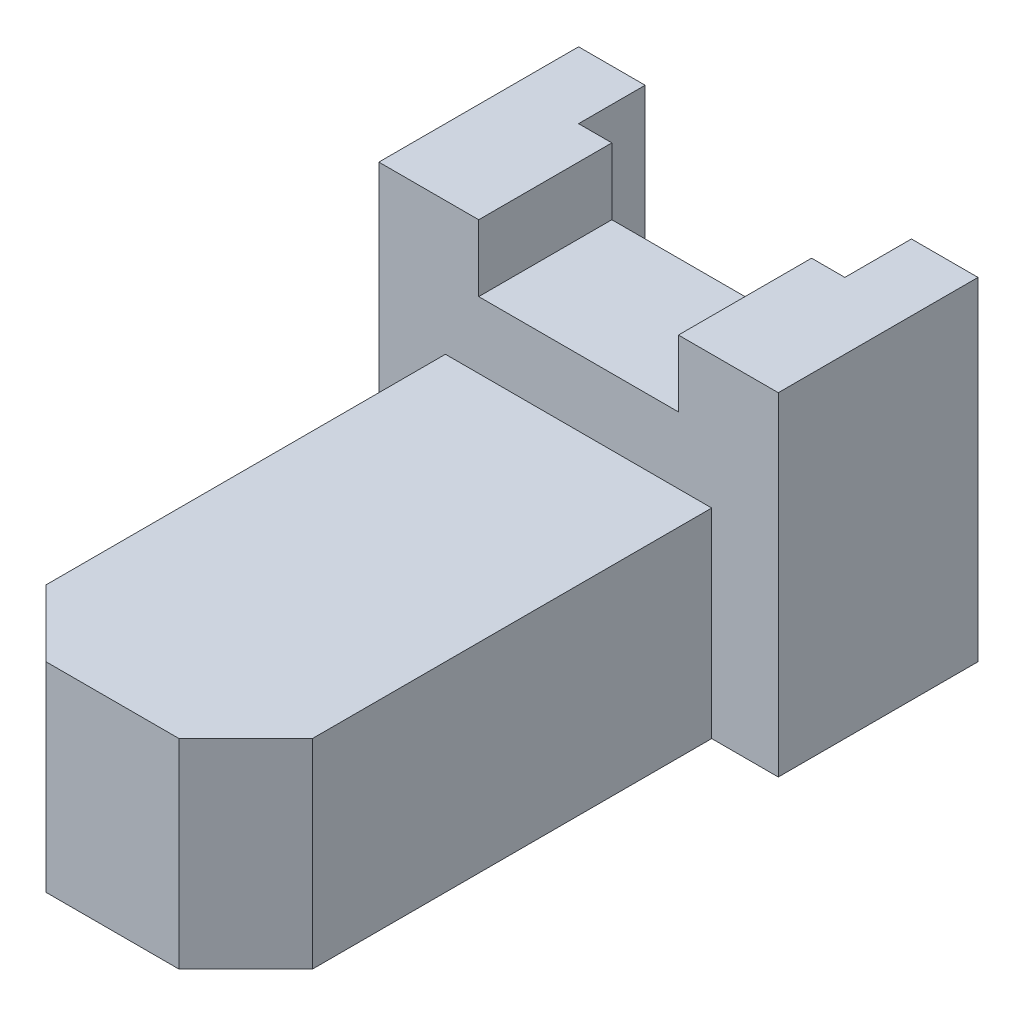
ISO-10303-21;
HEADER;
FILE_DESCRIPTION(('STEP AP214'),'2;1');
FILE_NAME('part.step','',(''),(''),'','','');
FILE_SCHEMA(('AUTOMOTIVE_DESIGN { 1 0 10303 214 1 1 1 1 }'));
ENDSEC;
DATA;
#1=APPLICATION_CONTEXT('core data for automotive mechanical design processes');
#2=APPLICATION_PROTOCOL_DEFINITION('international standard','automotive_design',2000,#1);
#3=PRODUCT_CONTEXT('',#1,'mechanical');
#4=PRODUCT('Part','Part','',(#3));
#5=PRODUCT_RELATED_PRODUCT_CATEGORY('part','',(#4));
#6=PRODUCT_DEFINITION_FORMATION('','',#4);
#7=PRODUCT_DEFINITION_CONTEXT('part definition',#1,'design');
#8=PRODUCT_DEFINITION('design','',#6,#7);
#9=PRODUCT_DEFINITION_SHAPE('','',#8);
#10=(LENGTH_UNIT() NAMED_UNIT(*) SI_UNIT(.MILLI.,.METRE.));
#11=(NAMED_UNIT(*) PLANE_ANGLE_UNIT() SI_UNIT($,.RADIAN.));
#12=(NAMED_UNIT(*) SI_UNIT($,.STERADIAN.) SOLID_ANGLE_UNIT());
#13=UNCERTAINTY_MEASURE_WITH_UNIT(LENGTH_MEASURE(1.E-05),#10,'distance_accuracy_value','');
#14=(GEOMETRIC_REPRESENTATION_CONTEXT(3) GLOBAL_UNCERTAINTY_ASSIGNED_CONTEXT((#13)) GLOBAL_UNIT_ASSIGNED_CONTEXT((#10,
#11,#12)) REPRESENTATION_CONTEXT('',''));
#15=CARTESIAN_POINT('',(0.,0.,0.));
#16=DIRECTION('',(0.,0.,1.));
#17=DIRECTION('',(1.,0.,0.));
#18=AXIS2_PLACEMENT_3D('',#15,#16,#17);
#19=CARTESIAN_POINT('',(0.,50.,0.));
#20=DIRECTION('',(0.,0.,-1.));
#21=DIRECTION('',(-1.,0.,0.));
#22=AXIS2_PLACEMENT_3D('',#19,#20,#21);
#23=PLANE('',#22);
#24=DIRECTION('',(0.,-1.,0.));
#25=VECTOR('',#24,1.);
#26=CARTESIAN_POINT('',(9.99999999999999,30.,0.));
#27=LINE('',#26,#25);
#28=CARTESIAN_POINT('',(9.99999999999999,30.,0.));
#29=VERTEX_POINT('',#28);
#30=CARTESIAN_POINT('',(9.99999999999999,0.,0.));
#31=VERTEX_POINT('',#30);
#32=EDGE_CURVE('E184',#29,#31,#27,.T.);
#33=ORIENTED_EDGE('',*,*,#32,.F.);
#34=DIRECTION('',(1.,0.,0.));
#35=VECTOR('',#34,1.);
#36=CARTESIAN_POINT('',(9.99999999999999,30.,0.));
#37=LINE('',#36,#35);
#38=CARTESIAN_POINT('',(50.,30.,0.));
#39=VERTEX_POINT('',#38);
#40=EDGE_CURVE('E188',#29,#39,#37,.T.);
#41=ORIENTED_EDGE('',*,*,#40,.T.);
#42=DIRECTION('',(0.,-1.,0.));
#43=VECTOR('',#42,1.);
#44=CARTESIAN_POINT('',(50.,30.,0.));
#45=LINE('',#44,#43);
#46=CARTESIAN_POINT('',(50.,0.,0.));
#47=VERTEX_POINT('',#46);
#48=EDGE_CURVE('E190',#39,#47,#45,.T.);
#49=ORIENTED_EDGE('',*,*,#48,.T.);
#50=DIRECTION('',(1.,0.,0.));
#51=VECTOR('',#50,1.);
#52=CARTESIAN_POINT('',(0.,0.,0.));
#53=LINE('',#52,#51);
#54=CARTESIAN_POINT('',(60.,0.,0.));
#55=VERTEX_POINT('',#54);
#56=EDGE_CURVE('E249',#47,#55,#53,.T.);
#57=ORIENTED_EDGE('',*,*,#56,.T.);
#58=DIRECTION('',(0.,-1.,0.));
#59=VECTOR('',#58,1.);
#60=CARTESIAN_POINT('',(60.,50.,0.));
#61=LINE('',#60,#59);
#62=CARTESIAN_POINT('',(60.,50.,0.));
#63=VERTEX_POINT('',#62);
#64=EDGE_CURVE('E279',#63,#55,#61,.T.);
#65=ORIENTED_EDGE('',*,*,#64,.F.);
#66=DIRECTION('',(1.,0.,0.));
#67=VECTOR('',#66,1.);
#68=CARTESIAN_POINT('',(0.,50.,0.));
#69=LINE('',#68,#67);
#70=CARTESIAN_POINT('',(45.,50.,0.));
#71=VERTEX_POINT('',#70);
#72=EDGE_CURVE('E226',#71,#63,#69,.T.);
#73=ORIENTED_EDGE('',*,*,#72,.F.);
#74=DIRECTION('',(0.,-1.,0.));
#75=VECTOR('',#74,1.);
#76=CARTESIAN_POINT('',(45.,50.,0.));
#77=LINE('',#76,#75);
#78=CARTESIAN_POINT('',(45.,40.,0.));
#79=VERTEX_POINT('',#78);
#80=EDGE_CURVE('E220',#71,#79,#77,.T.);
#81=ORIENTED_EDGE('',*,*,#80,.T.);
#82=DIRECTION('',(1.,0.,0.));
#83=VECTOR('',#82,1.);
#84=CARTESIAN_POINT('',(0.,40.,0.));
#85=LINE('',#84,#83);
#86=CARTESIAN_POINT('',(15.,40.,0.));
#87=VERTEX_POINT('',#86);
#88=EDGE_CURVE('E219',#87,#79,#85,.T.);
#89=ORIENTED_EDGE('',*,*,#88,.F.);
#90=DIRECTION('',(0.,-1.,0.));
#91=VECTOR('',#90,1.);
#92=CARTESIAN_POINT('',(15.,50.,0.));
#93=LINE('',#92,#91);
#94=CARTESIAN_POINT('',(15.,50.,0.));
#95=VERTEX_POINT('',#94);
#96=EDGE_CURVE('E213',#95,#87,#93,.T.);
#97=ORIENTED_EDGE('',*,*,#96,.F.);
#98=CARTESIAN_POINT('',(0.,50.,0.));
#99=VERTEX_POINT('',#98);
#100=EDGE_CURVE('E228',#99,#95,#69,.T.);
#101=ORIENTED_EDGE('',*,*,#100,.F.);
#102=DIRECTION('',(0.,-1.,0.));
#103=VECTOR('',#102,1.);
#104=CARTESIAN_POINT('',(0.,50.,0.));
#105=LINE('',#104,#103);
#106=CARTESIAN_POINT('',(0.,0.,0.));
#107=VERTEX_POINT('',#106);
#108=EDGE_CURVE('E282',#99,#107,#105,.T.);
#109=ORIENTED_EDGE('',*,*,#108,.T.);
#110=EDGE_CURVE('E253',#107,#31,#53,.T.);
#111=ORIENTED_EDGE('',*,*,#110,.T.);
#112=EDGE_LOOP('',(#33,#41,#49,#57,#65,#73,#81,#89,#97,#101,#109,#111));
#113=FACE_BOUND('',#112,.T.);
#114=ADVANCED_FACE('F41',(#113),#23,.F.);
#115=CARTESIAN_POINT('',(0.,50.,0.));
#116=DIRECTION('',(0.,1.,0.));
#117=DIRECTION('',(0.,0.,1.));
#118=AXIS2_PLACEMENT_3D('',#115,#116,#117);
#119=PLANE('',#118);
#120=ORIENTED_EDGE('',*,*,#100,.T.);
#121=DIRECTION('',(0.,0.,-1.));
#122=VECTOR('',#121,1.);
#123=CARTESIAN_POINT('',(15.,50.,0.));
#124=LINE('',#123,#122);
#125=CARTESIAN_POINT('',(15.,50.,-20.));
#126=VERTEX_POINT('',#125);
#127=EDGE_CURVE('E47',#95,#126,#124,.T.);
#128=ORIENTED_EDGE('',*,*,#127,.T.);
#129=DIRECTION('',(-1.,0.,0.));
#130=VECTOR('',#129,1.);
#131=CARTESIAN_POINT('',(50.,50.,-20.));
#132=LINE('',#131,#130);
#133=CARTESIAN_POINT('',(10.,50.,-20.));
#134=VERTEX_POINT('',#133);
#135=EDGE_CURVE('E239',#126,#134,#132,.T.);
#136=ORIENTED_EDGE('',*,*,#135,.T.);
#137=DIRECTION('',(0.,0.,-1.));
#138=VECTOR('',#137,1.);
#139=CARTESIAN_POINT('',(10.,50.,-20.));
#140=LINE('',#139,#138);
#141=CARTESIAN_POINT('',(10.,50.,-30.));
#142=VERTEX_POINT('',#141);
#143=EDGE_CURVE('E245',#134,#142,#140,.T.);
#144=ORIENTED_EDGE('',*,*,#143,.T.);
#145=DIRECTION('',(-1.,0.,0.));
#146=VECTOR('',#145,1.);
#147=CARTESIAN_POINT('',(10.,50.,-30.));
#148=LINE('',#147,#146);
#149=CARTESIAN_POINT('',(0.,50.,-30.));
#150=VERTEX_POINT('',#149);
#151=EDGE_CURVE('E224',#142,#150,#148,.T.);
#152=ORIENTED_EDGE('',*,*,#151,.T.);
#153=DIRECTION('',(0.,0.,1.));
#154=VECTOR('',#153,1.);
#155=CARTESIAN_POINT('',(0.,50.,-30.));
#156=LINE('',#155,#154);
#157=EDGE_CURVE('E227',#150,#99,#156,.T.);
#158=ORIENTED_EDGE('',*,*,#157,.T.);
#159=EDGE_LOOP('',(#120,#128,#136,#144,#152,#158));
#160=FACE_BOUND('',#159,.T.);
#161=ADVANCED_FACE('F287',(#160),#119,.T.);
#162=CARTESIAN_POINT('',(10.,50.,-30.));
#163=DIRECTION('',(0.,0.,1.));
#164=DIRECTION('',(1.,0.,0.));
#165=AXIS2_PLACEMENT_3D('',#162,#163,#164);
#166=PLANE('',#165);
#167=DIRECTION('',(-1.,0.,0.));
#168=VECTOR('',#167,1.);
#169=CARTESIAN_POINT('',(10.,0.,-30.));
#170=LINE('',#169,#168);
#171=CARTESIAN_POINT('',(10.,0.,-30.));
#172=VERTEX_POINT('',#171);
#173=CARTESIAN_POINT('',(0.,0.,-30.));
#174=VERTEX_POINT('',#173);
#175=EDGE_CURVE('E225',#172,#174,#170,.T.);
#176=ORIENTED_EDGE('',*,*,#175,.T.);
#177=DIRECTION('',(0.,-1.,0.));
#178=VECTOR('',#177,1.);
#179=CARTESIAN_POINT('',(0.,50.,-30.));
#180=LINE('',#179,#178);
#181=EDGE_CURVE('E281',#150,#174,#180,.T.);
#182=ORIENTED_EDGE('',*,*,#181,.F.);
#183=ORIENTED_EDGE('',*,*,#151,.F.);
#184=DIRECTION('',(0.,-1.,0.));
#185=VECTOR('',#184,1.);
#186=CARTESIAN_POINT('',(10.,50.,-30.));
#187=LINE('',#186,#185);
#188=EDGE_CURVE('E243',#142,#172,#187,.T.);
#189=ORIENTED_EDGE('',*,*,#188,.T.);
#190=EDGE_LOOP('',(#176,#182,#183,#189));
#191=FACE_BOUND('',#190,.T.);
#192=ADVANCED_FACE('F43',(#191),#166,.F.);
#193=CARTESIAN_POINT('',(0.,50.,-30.));
#194=DIRECTION('',(1.,0.,0.));
#195=DIRECTION('',(0.,0.,-1.));
#196=AXIS2_PLACEMENT_3D('',#193,#194,#195);
#197=PLANE('',#196);
#198=DIRECTION('',(0.,0.,1.));
#199=VECTOR('',#198,1.);
#200=CARTESIAN_POINT('',(0.,0.,-30.));
#201=LINE('',#200,#199);
#202=EDGE_CURVE('E246',#174,#107,#201,.T.);
#203=ORIENTED_EDGE('',*,*,#202,.T.);
#204=ORIENTED_EDGE('',*,*,#108,.F.);
#205=ORIENTED_EDGE('',*,*,#157,.F.);
#206=ORIENTED_EDGE('',*,*,#181,.T.);
#207=EDGE_LOOP('',(#203,#204,#205,#206));
#208=FACE_BOUND('',#207,.T.);
#209=ADVANCED_FACE('F310',(#208),#197,.F.);
#210=CARTESIAN_POINT('',(60.,50.,0.));
#211=DIRECTION('',(-1.,0.,0.));
#212=DIRECTION('',(0.,0.,1.));
#213=AXIS2_PLACEMENT_3D('',#210,#211,#212);
#214=PLANE('',#213);
#215=DIRECTION('',(0.,0.,-1.));
#216=VECTOR('',#215,1.);
#217=CARTESIAN_POINT('',(60.,0.,0.));
#218=LINE('',#217,#216);
#219=CARTESIAN_POINT('',(60.,0.,-30.));
#220=VERTEX_POINT('',#219);
#221=EDGE_CURVE('E255',#55,#220,#218,.T.);
#222=ORIENTED_EDGE('',*,*,#221,.T.);
#223=DIRECTION('',(0.,-1.,0.));
#224=VECTOR('',#223,1.);
#225=CARTESIAN_POINT('',(60.,50.,-30.));
#226=LINE('',#225,#224);
#227=CARTESIAN_POINT('',(60.,50.,-30.));
#228=VERTEX_POINT('',#227);
#229=EDGE_CURVE('E274',#228,#220,#226,.T.);
#230=ORIENTED_EDGE('',*,*,#229,.F.);
#231=DIRECTION('',(0.,0.,-1.));
#232=VECTOR('',#231,1.);
#233=CARTESIAN_POINT('',(60.,50.,0.));
#234=LINE('',#233,#232);
#235=EDGE_CURVE('E231',#63,#228,#234,.T.);
#236=ORIENTED_EDGE('',*,*,#235,.F.);
#237=ORIENTED_EDGE('',*,*,#64,.T.);
#238=EDGE_LOOP('',(#222,#230,#236,#237));
#239=FACE_BOUND('',#238,.T.);
#240=ADVANCED_FACE('F357',(#239),#214,.F.);
#241=CARTESIAN_POINT('',(60.,50.,-30.));
#242=DIRECTION('',(0.,0.,1.));
#243=DIRECTION('',(1.,0.,0.));
#244=AXIS2_PLACEMENT_3D('',#241,#242,#243);
#245=PLANE('',#244);
#246=DIRECTION('',(-1.,0.,0.));
#247=VECTOR('',#246,1.);
#248=CARTESIAN_POINT('',(60.,0.,-30.));
#249=LINE('',#248,#247);
#250=CARTESIAN_POINT('',(50.,0.,-30.));
#251=VERTEX_POINT('',#250);
#252=EDGE_CURVE('E258',#220,#251,#249,.T.);
#253=ORIENTED_EDGE('',*,*,#252,.T.);
#254=DIRECTION('',(0.,-1.,0.));
#255=VECTOR('',#254,1.);
#256=CARTESIAN_POINT('',(50.,50.,-30.));
#257=LINE('',#256,#255);
#258=CARTESIAN_POINT('',(50.,50.,-30.));
#259=VERTEX_POINT('',#258);
#260=EDGE_CURVE('E275',#259,#251,#257,.T.);
#261=ORIENTED_EDGE('',*,*,#260,.F.);
#262=DIRECTION('',(-1.,0.,0.));
#263=VECTOR('',#262,1.);
#264=CARTESIAN_POINT('',(60.,50.,-30.));
#265=LINE('',#264,#263);
#266=EDGE_CURVE('E234',#228,#259,#265,.T.);
#267=ORIENTED_EDGE('',*,*,#266,.F.);
#268=ORIENTED_EDGE('',*,*,#229,.T.);
#269=EDGE_LOOP('',(#253,#261,#267,#268));
#270=FACE_BOUND('',#269,.T.);
#271=ADVANCED_FACE('F383',(#270),#245,.F.);
#272=CARTESIAN_POINT('',(50.,50.,-30.));
#273=DIRECTION('',(1.,0.,0.));
#274=DIRECTION('',(0.,0.,-1.));
#275=AXIS2_PLACEMENT_3D('',#272,#273,#274);
#276=PLANE('',#275);
#277=DIRECTION('',(0.,0.,1.));
#278=VECTOR('',#277,1.);
#279=CARTESIAN_POINT('',(50.,0.,-30.));
#280=LINE('',#279,#278);
#281=CARTESIAN_POINT('',(50.,0.,-20.));
#282=VERTEX_POINT('',#281);
#283=EDGE_CURVE('E256',#251,#282,#280,.T.);
#284=ORIENTED_EDGE('',*,*,#283,.T.);
#285=DIRECTION('',(0.,-1.,0.));
#286=VECTOR('',#285,1.);
#287=CARTESIAN_POINT('',(50.,50.,-20.));
#288=LINE('',#287,#286);
#289=CARTESIAN_POINT('',(50.,50.,-20.));
#290=VERTEX_POINT('',#289);
#291=EDGE_CURVE('E267',#290,#282,#288,.T.);
#292=ORIENTED_EDGE('',*,*,#291,.F.);
#293=DIRECTION('',(0.,0.,1.));
#294=VECTOR('',#293,1.);
#295=CARTESIAN_POINT('',(50.,50.,-30.));
#296=LINE('',#295,#294);
#297=EDGE_CURVE('E240',#259,#290,#296,.T.);
#298=ORIENTED_EDGE('',*,*,#297,.F.);
#299=ORIENTED_EDGE('',*,*,#260,.T.);
#300=EDGE_LOOP('',(#284,#292,#298,#299));
#301=FACE_BOUND('',#300,.T.);
#302=ADVANCED_FACE('F332',(#301),#276,.F.);
#303=CARTESIAN_POINT('',(26.1604584527221,50.,-20.));
#304=DIRECTION('',(0.,0.,1.));
#305=DIRECTION('',(1.,0.,0.));
#306=AXIS2_PLACEMENT_3D('',#303,#304,#305);
#307=PLANE('',#306);
#308=DIRECTION('',(-1.,0.,0.));
#309=VECTOR('',#308,1.);
#310=CARTESIAN_POINT('',(45.,40.,-20.));
#311=LINE('',#310,#309);
#312=CARTESIAN_POINT('',(45.,40.,-20.));
#313=VERTEX_POINT('',#312);
#314=CARTESIAN_POINT('',(15.,40.,-20.));
#315=VERTEX_POINT('',#314);
#316=EDGE_CURVE('E202',#313,#315,#311,.T.);
#317=ORIENTED_EDGE('',*,*,#316,.F.);
#318=DIRECTION('',(0.,1.,0.));
#319=VECTOR('',#318,1.);
#320=CARTESIAN_POINT('',(45.,40.,-20.));
#321=LINE('',#320,#319);
#322=CARTESIAN_POINT('',(45.,50.,-20.));
#323=VERTEX_POINT('',#322);
#324=EDGE_CURVE('E209',#313,#323,#321,.T.);
#325=ORIENTED_EDGE('',*,*,#324,.T.);
#326=EDGE_CURVE('E238',#290,#323,#132,.T.);
#327=ORIENTED_EDGE('',*,*,#326,.F.);
#328=ORIENTED_EDGE('',*,*,#291,.T.);
#329=DIRECTION('',(-1.,0.,0.));
#330=VECTOR('',#329,1.);
#331=CARTESIAN_POINT('',(26.1604584527221,0.,-20.));
#332=LINE('',#331,#330);
#333=CARTESIAN_POINT('',(10.,0.,-20.));
#334=VERTEX_POINT('',#333);
#335=EDGE_CURVE('E261',#282,#334,#332,.T.);
#336=ORIENTED_EDGE('',*,*,#335,.T.);
#337=DIRECTION('',(0.,-1.,0.));
#338=VECTOR('',#337,1.);
#339=CARTESIAN_POINT('',(10.,50.,-20.));
#340=LINE('',#339,#338);
#341=EDGE_CURVE('E266',#134,#334,#340,.T.);
#342=ORIENTED_EDGE('',*,*,#341,.F.);
#343=ORIENTED_EDGE('',*,*,#135,.F.);
#344=DIRECTION('',(0.,1.,0.));
#345=VECTOR('',#344,1.);
#346=CARTESIAN_POINT('',(15.,40.,-20.));
#347=LINE('',#346,#345);
#348=EDGE_CURVE('E211',#315,#126,#347,.T.);
#349=ORIENTED_EDGE('',*,*,#348,.F.);
#350=EDGE_LOOP('',(#317,#325,#327,#328,#336,#342,#343,#349));
#351=FACE_BOUND('',#350,.T.);
#352=ADVANCED_FACE('F299',(#351),#307,.F.);
#353=CARTESIAN_POINT('',(10.,50.,-20.));
#354=DIRECTION('',(-1.,0.,0.));
#355=DIRECTION('',(0.,0.,1.));
#356=AXIS2_PLACEMENT_3D('',#353,#354,#355);
#357=PLANE('',#356);
#358=DIRECTION('',(0.,0.,-1.));
#359=VECTOR('',#358,1.);
#360=CARTESIAN_POINT('',(10.,0.,-20.));
#361=LINE('',#360,#359);
#362=EDGE_CURVE('E229',#334,#172,#361,.T.);
#363=ORIENTED_EDGE('',*,*,#362,.T.);
#364=ORIENTED_EDGE('',*,*,#188,.F.);
#365=ORIENTED_EDGE('',*,*,#143,.F.);
#366=ORIENTED_EDGE('',*,*,#341,.T.);
#367=EDGE_LOOP('',(#363,#364,#365,#366));
#368=FACE_BOUND('',#367,.T.);
#369=ADVANCED_FACE('F305',(#368),#357,.F.);
#370=DIRECTION('',(0.,0.,-1.));
#371=VECTOR('',#370,1.);
#372=CARTESIAN_POINT('',(45.,50.,0.));
#373=LINE('',#372,#371);
#374=EDGE_CURVE('E11',#71,#323,#373,.T.);
#375=ORIENTED_EDGE('',*,*,#374,.F.);
#376=ORIENTED_EDGE('',*,*,#72,.T.);
#377=ORIENTED_EDGE('',*,*,#235,.T.);
#378=ORIENTED_EDGE('',*,*,#266,.T.);
#379=ORIENTED_EDGE('',*,*,#297,.T.);
#380=ORIENTED_EDGE('',*,*,#326,.T.);
#381=EDGE_LOOP('',(#375,#376,#377,#378,#379,#380));
#382=FACE_BOUND('',#381,.T.);
#383=ADVANCED_FACE('F322',(#382),#119,.T.);
#384=CARTESIAN_POINT('',(0.,0.,0.));
#385=DIRECTION('',(0.,1.,0.));
#386=DIRECTION('',(0.,0.,1.));
#387=AXIS2_PLACEMENT_3D('',#384,#385,#386);
#388=PLANE('',#387);
#389=DIRECTION('',(0.,0.,1.));
#390=VECTOR('',#389,1.);
#391=CARTESIAN_POINT('',(50.,0.,0.));
#392=LINE('',#391,#390);
#393=CARTESIAN_POINT('',(50.,0.,60.));
#394=VERTEX_POINT('',#393);
#395=EDGE_CURVE('E198',#47,#394,#392,.T.);
#396=ORIENTED_EDGE('',*,*,#395,.T.);
#397=DIRECTION('',(0.707106781186548,0.,-0.707106781186548));
#398=VECTOR('',#397,1.);
#399=CARTESIAN_POINT('',(50.,0.,60.));
#400=LINE('',#399,#398);
#401=CARTESIAN_POINT('',(40.,0.,70.));
#402=VERTEX_POINT('',#401);
#403=EDGE_CURVE('E172',#402,#394,#400,.T.);
#404=ORIENTED_EDGE('',*,*,#403,.F.);
#405=DIRECTION('',(-1.,0.,0.));
#406=VECTOR('',#405,1.);
#407=CARTESIAN_POINT('',(9.99999999999999,0.,70.));
#408=LINE('',#407,#406);
#409=CARTESIAN_POINT('',(20.,0.,70.));
#410=VERTEX_POINT('',#409);
#411=EDGE_CURVE('E177',#402,#410,#408,.T.);
#412=ORIENTED_EDGE('',*,*,#411,.T.);
#413=DIRECTION('',(0.707106781186548,0.,0.707106781186548));
#414=VECTOR('',#413,1.);
#415=CARTESIAN_POINT('',(9.99999999999999,0.,60.));
#416=LINE('',#415,#414);
#417=CARTESIAN_POINT('',(9.99999999999999,0.,60.));
#418=VERTEX_POINT('',#417);
#419=EDGE_CURVE('E346',#418,#410,#416,.T.);
#420=ORIENTED_EDGE('',*,*,#419,.F.);
#421=DIRECTION('',(0.,0.,-1.));
#422=VECTOR('',#421,1.);
#423=CARTESIAN_POINT('',(9.99999999999999,0.,0.));
#424=LINE('',#423,#422);
#425=EDGE_CURVE('E192',#418,#31,#424,.T.);
#426=ORIENTED_EDGE('',*,*,#425,.T.);
#427=ORIENTED_EDGE('',*,*,#110,.F.);
#428=ORIENTED_EDGE('',*,*,#202,.F.);
#429=ORIENTED_EDGE('',*,*,#175,.F.);
#430=ORIENTED_EDGE('',*,*,#362,.F.);
#431=ORIENTED_EDGE('',*,*,#335,.F.);
#432=ORIENTED_EDGE('',*,*,#283,.F.);
#433=ORIENTED_EDGE('',*,*,#252,.F.);
#434=ORIENTED_EDGE('',*,*,#221,.F.);
#435=ORIENTED_EDGE('',*,*,#56,.F.);
#436=EDGE_LOOP('',(#396,#404,#412,#420,#426,#427,#428,#429,#430,#431,#432,#433,#434,#435));
#437=FACE_BOUND('',#436,.T.);
#438=ADVANCED_FACE('F333',(#437),#388,.F.);
#439=CARTESIAN_POINT('',(0.,40.,0.));
#440=DIRECTION('',(0.,1.,0.));
#441=DIRECTION('',(0.,0.,1.));
#442=AXIS2_PLACEMENT_3D('',#439,#440,#441);
#443=PLANE('',#442);
#444=ORIENTED_EDGE('',*,*,#88,.T.);
#445=DIRECTION('',(0.,0.,-1.));
#446=VECTOR('',#445,1.);
#447=CARTESIAN_POINT('',(45.,40.,20.));
#448=LINE('',#447,#446);
#449=EDGE_CURVE('E205',#79,#313,#448,.T.);
#450=ORIENTED_EDGE('',*,*,#449,.T.);
#451=ORIENTED_EDGE('',*,*,#316,.T.);
#452=DIRECTION('',(0.,0.,-1.));
#453=VECTOR('',#452,1.);
#454=CARTESIAN_POINT('',(15.,40.,20.));
#455=LINE('',#454,#453);
#456=EDGE_CURVE('E208',#87,#315,#455,.T.);
#457=ORIENTED_EDGE('',*,*,#456,.F.);
#458=EDGE_LOOP('',(#444,#450,#451,#457));
#459=FACE_BOUND('',#458,.T.);
#460=ADVANCED_FACE('F320',(#459),#443,.T.);
#461=CARTESIAN_POINT('',(45.,40.,20.));
#462=DIRECTION('',(1.,0.,0.));
#463=DIRECTION('',(0.,0.,-1.));
#464=AXIS2_PLACEMENT_3D('',#461,#462,#463);
#465=PLANE('',#464);
#466=ORIENTED_EDGE('',*,*,#374,.T.);
#467=ORIENTED_EDGE('',*,*,#324,.F.);
#468=ORIENTED_EDGE('',*,*,#449,.F.);
#469=ORIENTED_EDGE('',*,*,#80,.F.);
#470=EDGE_LOOP('',(#466,#467,#468,#469));
#471=FACE_BOUND('',#470,.T.);
#472=ADVANCED_FACE('F363',(#471),#465,.F.);
#473=CARTESIAN_POINT('',(15.,40.,20.));
#474=DIRECTION('',(1.,0.,0.));
#475=DIRECTION('',(0.,0.,-1.));
#476=AXIS2_PLACEMENT_3D('',#473,#474,#475);
#477=PLANE('',#476);
#478=ORIENTED_EDGE('',*,*,#96,.T.);
#479=ORIENTED_EDGE('',*,*,#456,.T.);
#480=ORIENTED_EDGE('',*,*,#348,.T.);
#481=ORIENTED_EDGE('',*,*,#127,.F.);
#482=EDGE_LOOP('',(#478,#479,#480,#481));
#483=FACE_BOUND('',#482,.T.);
#484=ADVANCED_FACE('F312',(#483),#477,.T.);
#485=CARTESIAN_POINT('',(9.99999999999999,30.,0.));
#486=DIRECTION('',(-1.,0.,0.));
#487=DIRECTION('',(0.,0.,1.));
#488=AXIS2_PLACEMENT_3D('',#485,#486,#487);
#489=PLANE('',#488);
#490=DIRECTION('',(0.,-1.,0.));
#491=VECTOR('',#490,1.);
#492=CARTESIAN_POINT('',(9.99999999999999,30.,60.));
#493=LINE('',#492,#491);
#494=CARTESIAN_POINT('',(9.99999999999999,30.,60.));
#495=VERTEX_POINT('',#494);
#496=EDGE_CURVE('E342',#495,#418,#493,.T.);
#497=ORIENTED_EDGE('',*,*,#496,.F.);
#498=DIRECTION('',(0.,0.,-1.));
#499=VECTOR('',#498,1.);
#500=CARTESIAN_POINT('',(9.99999999999999,30.,0.));
#501=LINE('',#500,#499);
#502=EDGE_CURVE('E199',#495,#29,#501,.T.);
#503=ORIENTED_EDGE('',*,*,#502,.T.);
#504=ORIENTED_EDGE('',*,*,#32,.T.);
#505=ORIENTED_EDGE('',*,*,#425,.F.);
#506=EDGE_LOOP('',(#497,#503,#504,#505));
#507=FACE_BOUND('',#506,.T.);
#508=ADVANCED_FACE('F341',(#507),#489,.T.);
#509=CARTESIAN_POINT('',(9.99999999999999,30.,70.));
#510=DIRECTION('',(0.,0.,1.));
#511=DIRECTION('',(1.,0.,0.));
#512=AXIS2_PLACEMENT_3D('',#509,#510,#511);
#513=PLANE('',#512);
#514=DIRECTION('',(0.,-1.,0.));
#515=VECTOR('',#514,1.);
#516=CARTESIAN_POINT('',(40.,30.,70.));
#517=LINE('',#516,#515);
#518=CARTESIAN_POINT('',(40.,30.,70.));
#519=VERTEX_POINT('',#518);
#520=EDGE_CURVE('E164',#519,#402,#517,.T.);
#521=ORIENTED_EDGE('',*,*,#520,.F.);
#522=DIRECTION('',(-1.,0.,0.));
#523=VECTOR('',#522,1.);
#524=CARTESIAN_POINT('',(9.99999999999999,30.,70.));
#525=LINE('',#524,#523);
#526=CARTESIAN_POINT('',(20.,30.,70.));
#527=VERTEX_POINT('',#526);
#528=EDGE_CURVE('E180',#519,#527,#525,.T.);
#529=ORIENTED_EDGE('',*,*,#528,.T.);
#530=DIRECTION('',(0.,-1.,0.));
#531=VECTOR('',#530,1.);
#532=CARTESIAN_POINT('',(20.,30.,70.));
#533=LINE('',#532,#531);
#534=EDGE_CURVE('E61',#527,#410,#533,.T.);
#535=ORIENTED_EDGE('',*,*,#534,.T.);
#536=ORIENTED_EDGE('',*,*,#411,.F.);
#537=EDGE_LOOP('',(#521,#529,#535,#536));
#538=FACE_BOUND('',#537,.T.);
#539=ADVANCED_FACE('F178',(#538),#513,.T.);
#540=CARTESIAN_POINT('',(50.,30.,0.));
#541=DIRECTION('',(1.,0.,0.));
#542=DIRECTION('',(0.,0.,-1.));
#543=AXIS2_PLACEMENT_3D('',#540,#541,#542);
#544=PLANE('',#543);
#545=DIRECTION('',(0.,-1.,0.));
#546=VECTOR('',#545,1.);
#547=CARTESIAN_POINT('',(50.,30.,60.));
#548=LINE('',#547,#546);
#549=CARTESIAN_POINT('',(50.,30.,60.));
#550=VERTEX_POINT('',#549);
#551=EDGE_CURVE('E57',#550,#394,#548,.T.);
#552=ORIENTED_EDGE('',*,*,#551,.T.);
#553=ORIENTED_EDGE('',*,*,#395,.F.);
#554=ORIENTED_EDGE('',*,*,#48,.F.);
#555=DIRECTION('',(0.,0.,1.));
#556=VECTOR('',#555,1.);
#557=CARTESIAN_POINT('',(50.,30.,0.));
#558=LINE('',#557,#556);
#559=EDGE_CURVE('E183',#39,#550,#558,.T.);
#560=ORIENTED_EDGE('',*,*,#559,.T.);
#561=EDGE_LOOP('',(#552,#553,#554,#560));
#562=FACE_BOUND('',#561,.T.);
#563=ADVANCED_FACE('F351',(#562),#544,.T.);
#564=CARTESIAN_POINT('',(0.,30.,0.));
#565=DIRECTION('',(0.,1.,0.));
#566=DIRECTION('',(0.,0.,1.));
#567=AXIS2_PLACEMENT_3D('',#564,#565,#566);
#568=PLANE('',#567);
#569=DIRECTION('',(0.707106781186548,0.,-0.707106781186548));
#570=VECTOR('',#569,1.);
#571=CARTESIAN_POINT('',(50.,30.,60.));
#572=LINE('',#571,#570);
#573=EDGE_CURVE('E165',#519,#550,#572,.T.);
#574=ORIENTED_EDGE('',*,*,#573,.T.);
#575=ORIENTED_EDGE('',*,*,#559,.F.);
#576=ORIENTED_EDGE('',*,*,#40,.F.);
#577=ORIENTED_EDGE('',*,*,#502,.F.);
#578=DIRECTION('',(0.707106781186548,0.,0.707106781186548));
#579=VECTOR('',#578,1.);
#580=CARTESIAN_POINT('',(9.99999999999999,30.,60.));
#581=LINE('',#580,#579);
#582=EDGE_CURVE('E181',#495,#527,#581,.T.);
#583=ORIENTED_EDGE('',*,*,#582,.T.);
#584=ORIENTED_EDGE('',*,*,#528,.F.);
#585=EDGE_LOOP('',(#574,#575,#576,#577,#583,#584));
#586=FACE_BOUND('',#585,.T.);
#587=ADVANCED_FACE('F182',(#586),#568,.T.);
#588=CARTESIAN_POINT('',(9.99999999999999,30.,60.));
#589=DIRECTION('',(0.707106781186547,0.,-0.707106781186547));
#590=DIRECTION('',(-0.707106781186548,0.,-0.707106781186548));
#591=AXIS2_PLACEMENT_3D('',#588,#589,#590);
#592=PLANE('',#591);
#593=ORIENTED_EDGE('',*,*,#419,.T.);
#594=ORIENTED_EDGE('',*,*,#534,.F.);
#595=ORIENTED_EDGE('',*,*,#582,.F.);
#596=ORIENTED_EDGE('',*,*,#496,.T.);
#597=EDGE_LOOP('',(#593,#594,#595,#596));
#598=FACE_BOUND('',#597,.T.);
#599=ADVANCED_FACE('F505',(#598),#592,.F.);
#600=CARTESIAN_POINT('',(50.,30.,60.));
#601=DIRECTION('',(-0.707106781186547,0.,-0.707106781186547));
#602=DIRECTION('',(-0.707106781186548,0.,0.707106781186548));
#603=AXIS2_PLACEMENT_3D('',#600,#601,#602);
#604=PLANE('',#603);
#605=ORIENTED_EDGE('',*,*,#403,.T.);
#606=ORIENTED_EDGE('',*,*,#551,.F.);
#607=ORIENTED_EDGE('',*,*,#573,.F.);
#608=ORIENTED_EDGE('',*,*,#520,.T.);
#609=EDGE_LOOP('',(#605,#606,#607,#608));
#610=FACE_BOUND('',#609,.T.);
#611=ADVANCED_FACE('F163',(#610),#604,.F.);
#612=CLOSED_SHELL('',(#114,#161,#192,#209,#240,#271,#302,#352,#369,#383,#438,#460,#472,#484,
#508,#539,#563,#587,#599,#611));
#613=MANIFOLD_SOLID_BREP('B2',#612);
#614=ADVANCED_BREP_SHAPE_REPRESENTATION('',(#18,#613),#14);
#615=SHAPE_DEFINITION_REPRESENTATION(#9,#614);
ENDSEC;
END-ISO-10303-21;
